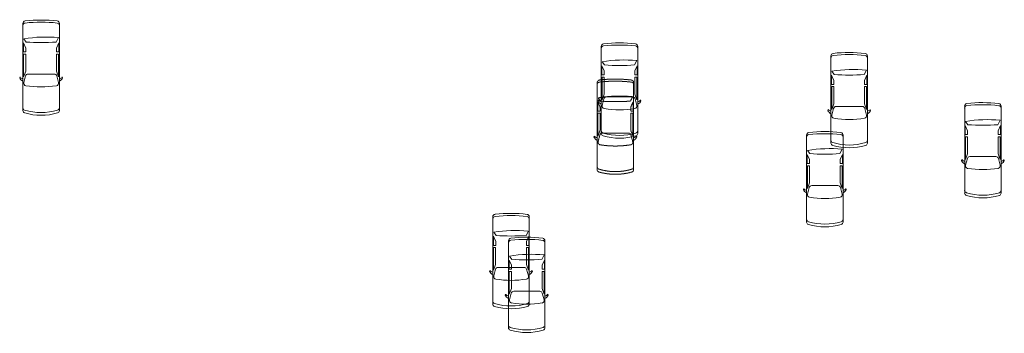
# Model space of a CAD drawing. Units: inches. Extents: x 79 to 8696167, y -3690578 to 147.
# Tile 8 of 10: x 219238 to 221194, y -94369 to -93746. Entities that reach past the tile are written whole.
import ezdxf

# ---------------------------------------------------------------- set-up
doc = ezdxf.new("R2010")
doc.units = ezdxf.units.IN
doc.header["$MEASUREMENT"] = 0
doc.linetypes.add('HIDDEN', pattern=[0.375, 0.25, -0.125])
for name, color, linetype, lineweight in [('C-PKNG-VEHI', 8, 'Continuous', 13), ('C-PKNG-VEHI-HIDN', 8, 'HIDDEN', 13), ('PLUMBING FIXTURES', 9, 'Continuous', 18)]:
    doc.layers.add(name, color=color, linetype=linetype, lineweight=lineweight)

# ---------------------------------------------------------------- blocks, each defined once
blk = doc.blocks.new('CAR')
at = {"layer": 'PLUMBING FIXTURES', "ltscale": 3}
for p, q in [((220804.5, -93720.1), (220804.5, -93547.3)), ((220876.9, -93720.1), (220876.9, -93547.3)), ((220810.2, -93596.1), (220805.6, -93585.7)), ((220805.6, -93585.7), (220805.6, -93603.9)), ((220810.8, -93584.2), (220806.3, -93577.8)), ((220870.5, -93584.2), (220875, -93575.4)), ((220871.1, -93596.1), (220875.8, -93585.7)), ((220875.8, -93585.7), (220875.8, -93603.9)), ((220805.6, -93603.9), (220810.2, -93603.9)), ((220806, -93608.1), (220810.1, -93608.1)), ((220806, -93653.3), (220806, -93608.1)), ((220810.1, -93608.1), (220810.1, -93642.1)), ((220810.2, -93603.9), (220810.2, -93596.1)), ((220871.1, -93603.9), (220871.1, -93596.1)), ((220875.8, -93603.9), (220871.1, -93603.9)), ((220875.3, -93608.1), (220871.2, -93608.1)), ((220871.2, -93608.1), (220871.2, -93642.1)), ((220875.3, -93653.3), (220875.3, -93608.1)), ((220810.1, -93642.1), (220806, -93653.3)), ((220814.7, -93647.6), (220866.7, -93647.6)), ((220871.2, -93642.1), (220875.3, -93653.3)), ((220798.8, -93653.5), (220798.1, -93655.1)), ((220806.3, -93664.6), (220809.8, -93651.4)), ((220875, -93664.6), (220871.6, -93651.4)), ((220882.5, -93653.5), (220883.2, -93655.1))]:
    blk.add_line(p, q, dxfattribs=at)
for centre, radius, start, end in [((220809.5, -93547.3), 5.05, 97.3566, 180), ((220809.5, -93551.4), 5.05, 97.3566, 180), ((220840.5, -93811.7), 271.3, 83.2311, 96.6925), ((220840.5, -93815.9), 271.3, 83.2311, 96.6925), ((220871.8, -93547.3), 5.05, 360, 82.5593), ((220871.8, -93551.5), 5.05, 360, 82.5593), ((220849.4, -93837), 262.8, 84.4202, 99.448), ((220840.7, -93184.1), 401.2, 265.7353, 274.2647), ((220814.7, -93652.7), 5.05, 90, 165.2564), ((220866.7, -93652.7), 5.05, 14.7436, 90), ((220809.4, -93651), 12, 199.7943, 245.6458), ((220804.9, -93649.7), 7.17, 212.3474, 266.7713), ((220811.2, -93665.9), 5.05, 165.2564, 260.0648), ((220870.2, -93665.9), 5.05, 279.9351, 14.7436), ((220876.5, -93649.7), 7.17, 273.2287, 327.6525), ((220871.9, -93651), 12, 294.3542, 340.2056), ((220840.7, -93484.8), 188.5, 260.7342, 279.2658), ((220809.5, -93714.4), 5.05, 180, 251.4636), ((220809.5, -93720.1), 5.05, 180, 252.5507), ((220840.7, -93611.6), 112.5, 253.0675, 286.9325), ((220840.7, -93610.5), 119, 254.0673, 285.9327), ((220871.8, -93720.1), 5.05, 287.4493, 360), ((220871.8, -93714.4), 5.05, 288.5363, 360)]:
    blk.add_arc(centre, radius, start, end, dxfattribs=at)

msp = doc.modelspace()

# ---------------------------------------------------------------- linework, layer by layer
at = {"layer": 'C-PKNG-VEHI-HIDN', "ltscale": 3}
for p, q in [((220385.025, -94043.911), (220385.025, -93871.153)), ((220457.415, -94043.911), (220457.415, -93871.194)), ((220391.386, -93908.015), (220386.863, -93901.607)), ((220451.054, -93908.015), (220455.555, -93899.287)), ((220390.78, -93919.929), (220386.136, -93909.53)), ((220386.136, -93909.53), (220386.136, -93927.703)), ((220390.78, -93927.703), (220390.78, -93919.929)), ((220451.66, -93919.929), (220456.304, -93909.53)), ((220451.66, -93927.703), (220451.66, -93919.929)), ((220456.304, -93909.53), (220456.304, -93927.703)), ((220386.136, -93927.703), (220390.78, -93927.703)), ((220386.54, -93931.943), (220390.679, -93931.943)), ((220386.54, -93977.134), (220386.54, -93931.943)), ((220390.679, -93931.943), (220390.679, -93965.927)), ((220456.304, -93927.703), (220451.66, -93927.703)), ((220455.901, -93931.943), (220451.761, -93931.943)), ((220451.761, -93931.943), (220451.761, -93965.927)), ((220455.901, -93977.134), (220455.901, -93931.943)), ((220379.371, -93977.336), (220378.665, -93978.951)), ((220390.679, -93965.927), (220386.54, -93977.134)), ((220386.855, -93988.455), (220390.332, -93975.243)), ((220395.214, -93971.48), (220447.227, -93971.48)), ((220451.761, -93965.927), (220455.901, -93977.134)), ((220455.585, -93988.455), (220452.108, -93975.243)), ((220463.069, -93977.336), (220463.776, -93978.951))]:
    msp.add_line(p, q, dxfattribs=at)
for centre, radius, start, end in [((220421.044, -94135.594), 271.296, 83.231063, 96.692501), ((220390.073, -93871.153), 5.048, 97.356614, 179.999992), ((220390.073, -93875.292), 5.048, 97.356614, 179.999992), ((220421.044, -94139.733), 271.296, 83.231063, 96.692501), ((220452.367, -93871.194), 5.048, 359.999992, 82.559346), ((220452.367, -93875.333), 5.048, 359.999992, 82.559346), ((220430.002, -94160.84), 262.798, 84.420191, 99.448016), ((220421.22, -93507.932), 401.194, 265.735331, 274.264654), ((220389.988, -93974.876), 12.034, 199.794346, 245.645816), ((220385.429, -93973.499), 7.17, 212.347436, 266.771313), ((220395.214, -93976.528), 5.048, 89.999992, 165.256429), ((220447.227, -93976.528), 5.048, 14.743555, 89.999992), ((220457.011, -93973.499), 7.17, 273.228672, 327.652549), ((220452.452, -93974.876), 12.034, 294.354168, 340.205639), ((220391.737, -93989.739), 5.048, 165.256429, 260.064841), ((220421.22, -93808.654), 188.518, 260.734182, 279.265803), ((220450.703, -93989.739), 5.048, 279.935144, 14.743555), ((220390.073, -94038.285), 5.048, 179.999992, 251.463649), ((220452.367, -94038.285), 5.048, 288.536336, 359.999992), ((220390.073, -94043.911), 5.048, 179.999992, 252.550683), ((220421.22, -93935.493), 112.453, 253.067464, 286.93252), ((220421.22, -93934.319), 118.978, 254.067313, 285.932671), ((220452.367, -94043.911), 5.048, 287.449301, 359.999992)]:
    msp.add_arc(centre, radius, start, end, dxfattribs=at)

# ---------------------------------------------------------------- block references
at = {"layer": 'C-PKNG-VEHI'}
for p in [(-1560.037, -206.661), (-411.319, -252.118), (44.861, -271.087), (310.363, -370.6), (-3.559, -428.061), (-626.714, -590.471), (-595.556, -637.84)]:
    msp.add_blockref('CAR', p, dxfattribs=at)

doc.saveas('drawing.dxf')
